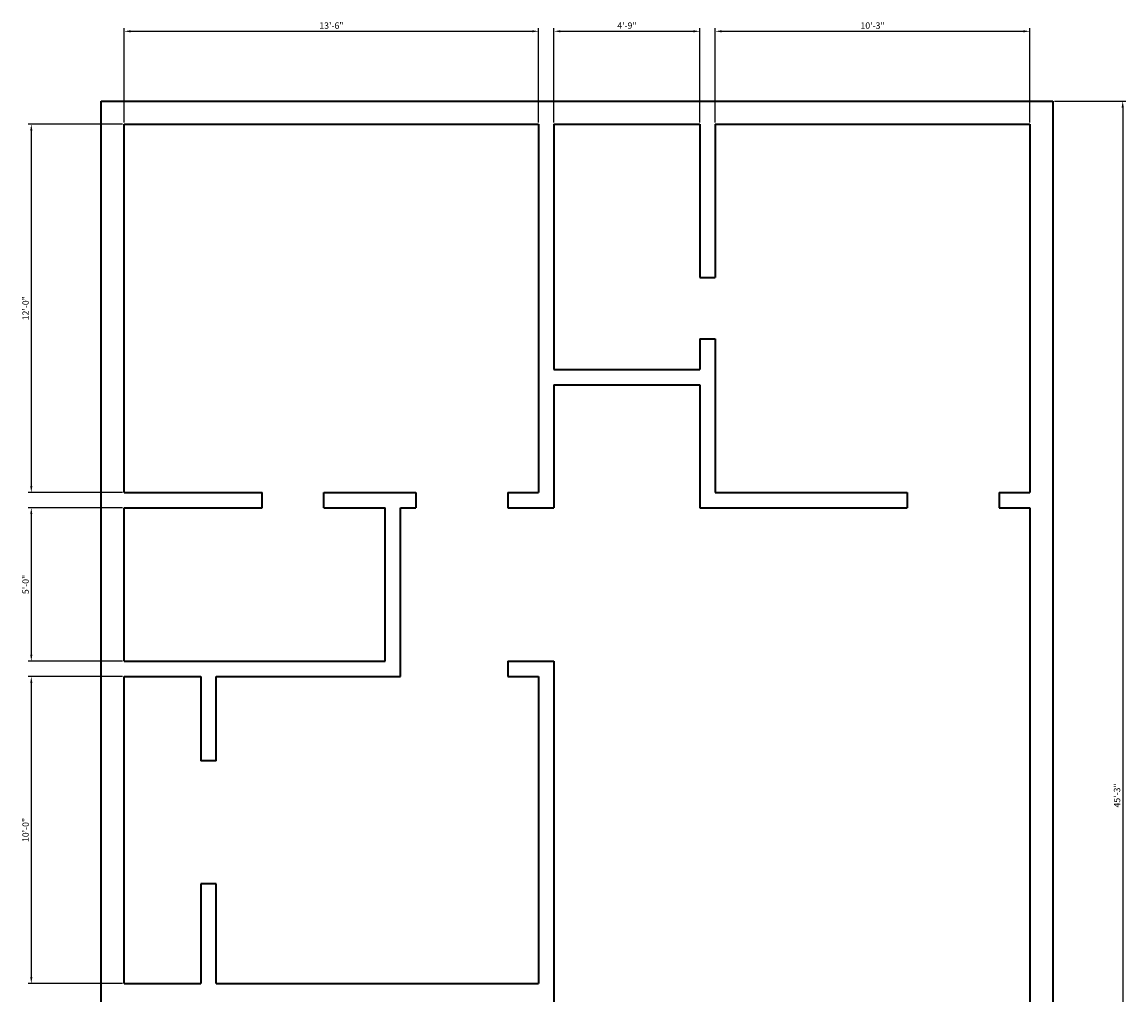
# Model space of a CAD drawing. Units: inches. Extents: x 2163 to 7246, y 928 to 2098.
# Tile 15 of 15: x 6815 to 7246, y 1625 to 2005. Entities that reach past the tile are written whole.
import ezdxf

# ---------------------------------------------------------------- set-up
doc = ezdxf.new("R2010")
doc.units = ezdxf.units.IN
doc.layers.add('A-ANNO-DIMS', color=4, linetype='Continuous', lineweight=18)
doc.layers.add('A-WALL', color=7, linetype='Continuous', lineweight=35)
doc.styles.get("Standard").update_dxf_attribs({"font": 'arial.ttf'})
doc.dimstyles.new('ISO-25', dxfattribs={"dimtxt": 2.5, "dimasz": 2.5, "dimexe": 1.25, "dimexo": 0.625, "dimtad": 1, "dimdec": 0, "dimlunit": 3, "dimtxsty": 'Standard', "dimcen": 2.5, "dimadec": 0, "dimazin": 0, "dimtfac": 1, "dimtdec": 0, "dimtmove": 0, "dimatfit": 3, "dimfxl": 1, "dimarcsym": 0})

# ---------------------------------------------------------------- blocks, each defined once
blk = doc.blocks.new('*D113')
at = {"layer": 'A-ANNO-DIMS', "color": 0, "lineweight": -2, "transparency": 16777216}
for p, q in [((7218.09, 1974.46), (7246.01, 1974.46)), ((7244.76, 1971.96), (7244.76, 1433.96)), ((7218.09, 1431.46), (7246.01, 1431.46))]:
    blk.add_line(p, q, dxfattribs=at)
at = {"layer": 'A-ANNO-DIMS', "color": 0, "transparency": 16777216}
for points in [[(7244.34, 1971.96), (7245.18, 1971.96), (7244.76, 1974.46)], [(7244.34, 1433.96), (7245.18, 1433.96), (7244.76, 1431.46)]]:
    blk.add_solid(points, dxfattribs=at)
at = {"layer": 'Defpoints', "color": 0, "transparency": 16777216}
for p in [(7217.46, 1974.46), (7217.46, 1431.46), (7244.76, 1431.46)]:
    blk.add_point(p, dxfattribs=at)
at = {"layer": 'A-ANNO-DIMS', "color": 0, "transparency": 16777216, "insert": (7242.86, 1702.96), "char_height": 2.5, "attachment_point": 5, "rotation": 90}
blk.add_mtext('45\'-3"', dxfattribs=at)
blk = doc.blocks.new('*D115')
at = {"layer": 'A-ANNO-DIMS', "color": 0, "lineweight": -2, "transparency": 16777216}
for p, q in [((6854.46, 1966.08), (6854.46, 2003.01)), ((7016.46, 1966.08), (7016.46, 2003.01)), ((6856.96, 2001.76), (7013.96, 2001.76))]:
    blk.add_line(p, q, dxfattribs=at)
at = {"layer": 'A-ANNO-DIMS', "color": 0, "transparency": 16777216}
for points in [[(6856.96, 2002.18), (6856.96, 2001.34), (6854.46, 2001.76)], [(7013.96, 2002.18), (7013.96, 2001.34), (7016.46, 2001.76)]]:
    blk.add_solid(points, dxfattribs=at)
at = {"layer": 'Defpoints', "color": 0, "transparency": 16777216}
for p in [(7016.46, 2001.76), (6854.46, 1965.46), (7016.46, 1965.46)]:
    blk.add_point(p, dxfattribs=at)
at = {"layer": 'A-ANNO-DIMS', "color": 0, "transparency": 16777216, "insert": (6935.46, 2003.66), "char_height": 2.5, "attachment_point": 5}
blk.add_mtext('13\'-6"', dxfattribs=at)
blk = doc.blocks.new('*D116')
at = {"layer": 'A-ANNO-DIMS', "color": 0, "lineweight": -2, "transparency": 16777216}
for p, q in [((7022.46, 1966.08), (7022.46, 2003.01)), ((7079.46, 1966.08), (7079.46, 2003.01)), ((7024.96, 2001.76), (7076.96, 2001.76))]:
    blk.add_line(p, q, dxfattribs=at)
at = {"layer": 'A-ANNO-DIMS', "color": 0, "transparency": 16777216}
for points in [[(7024.96, 2002.18), (7024.96, 2001.34), (7022.46, 2001.76)], [(7076.96, 2002.18), (7076.96, 2001.34), (7079.46, 2001.76)]]:
    blk.add_solid(points, dxfattribs=at)
at = {"layer": 'Defpoints', "color": 0, "transparency": 16777216}
for p in [(7079.46, 2001.76), (7022.46, 1965.46), (7079.46, 1965.46)]:
    blk.add_point(p, dxfattribs=at)
at = {"layer": 'A-ANNO-DIMS', "color": 0, "transparency": 16777216, "insert": (7050.96, 2003.66), "char_height": 2.5, "attachment_point": 5}
blk.add_mtext('4\'-9"', dxfattribs=at)
blk = doc.blocks.new('*D117')
at = {"layer": 'A-ANNO-DIMS', "color": 0, "lineweight": -2, "transparency": 16777216}
for p, q in [((7085.46, 1966.08), (7085.46, 2003.01)), ((7208.46, 1966.08), (7208.46, 2003.01)), ((7087.96, 2001.76), (7205.96, 2001.76))]:
    blk.add_line(p, q, dxfattribs=at)
at = {"layer": 'A-ANNO-DIMS', "color": 0, "transparency": 16777216}
for points in [[(7087.96, 2002.18), (7087.96, 2001.34), (7085.46, 2001.76)], [(7205.96, 2002.18), (7205.96, 2001.34), (7208.46, 2001.76)]]:
    blk.add_solid(points, dxfattribs=at)
at = {"layer": 'Defpoints', "color": 0, "transparency": 16777216}
for p in [(7208.46, 2001.76), (7085.46, 1965.46), (7208.46, 1965.46)]:
    blk.add_point(p, dxfattribs=at)
at = {"layer": 'A-ANNO-DIMS', "color": 0, "transparency": 16777216, "insert": (7146.96, 2003.66), "char_height": 2.5, "attachment_point": 5}
blk.add_mtext('10\'-3"', dxfattribs=at)
blk = doc.blocks.new('*D118')
at = {"layer": 'A-ANNO-DIMS', "color": 0, "lineweight": -2, "transparency": 16777216}
for p, q in [((6853.84, 1965.46), (6816.91, 1965.46)), ((6818.16, 1962.96), (6818.16, 1823.96)), ((6853.84, 1821.46), (6816.91, 1821.46))]:
    blk.add_line(p, q, dxfattribs=at)
at = {"layer": 'A-ANNO-DIMS', "color": 0, "transparency": 16777216}
for points in [[(6817.74, 1962.96), (6818.58, 1962.96), (6818.16, 1965.46)], [(6817.74, 1823.96), (6818.58, 1823.96), (6818.16, 1821.46)]]:
    blk.add_solid(points, dxfattribs=at)
at = {"layer": 'Defpoints', "color": 0, "transparency": 16777216}
for p in [(6854.46, 1965.46), (6818.16, 1821.46), (6854.46, 1821.46)]:
    blk.add_point(p, dxfattribs=at)
at = {"layer": 'A-ANNO-DIMS', "color": 0, "transparency": 16777216, "insert": (6816.26, 1893.46), "char_height": 2.5, "attachment_point": 5, "rotation": 90}
blk.add_mtext('12\'-0"', dxfattribs=at)
blk = doc.blocks.new('*D119')
at = {"layer": 'A-ANNO-DIMS', "color": 0, "lineweight": -2, "transparency": 16777216}
for p, q in [((6853.84, 1815.46), (6816.91, 1815.46)), ((6818.16, 1812.96), (6818.16, 1757.96)), ((6853.84, 1755.46), (6816.91, 1755.46))]:
    blk.add_line(p, q, dxfattribs=at)
at = {"layer": 'A-ANNO-DIMS', "color": 0, "transparency": 16777216}
for points in [[(6817.74, 1812.96), (6818.58, 1812.96), (6818.16, 1815.46)], [(6817.74, 1757.96), (6818.58, 1757.96), (6818.16, 1755.46)]]:
    blk.add_solid(points, dxfattribs=at)
at = {"layer": 'Defpoints', "color": 0, "transparency": 16777216}
for p in [(6854.46, 1815.46), (6818.16, 1755.46), (6854.46, 1755.46)]:
    blk.add_point(p, dxfattribs=at)
at = {"layer": 'A-ANNO-DIMS', "color": 0, "transparency": 16777216, "insert": (6816.26, 1785.46), "char_height": 2.5, "attachment_point": 5, "rotation": 90}
blk.add_mtext('5\'-0"', dxfattribs=at)
blk = doc.blocks.new('*D120')
at = {"layer": 'A-ANNO-DIMS', "color": 0, "lineweight": -2, "transparency": 16777216}
for p, q in [((6853.84, 1749.46), (6816.91, 1749.46)), ((6818.16, 1746.96), (6818.16, 1631.96)), ((6853.84, 1629.46), (6816.91, 1629.46))]:
    blk.add_line(p, q, dxfattribs=at)
at = {"layer": 'A-ANNO-DIMS', "color": 0, "transparency": 16777216}
for points in [[(6817.74, 1746.96), (6818.58, 1746.96), (6818.16, 1749.46)], [(6817.74, 1631.96), (6818.58, 1631.96), (6818.16, 1629.46)]]:
    blk.add_solid(points, dxfattribs=at)
at = {"layer": 'Defpoints', "color": 0, "transparency": 16777216}
for p in [(6854.46, 1749.46), (6818.16, 1629.46), (6854.46, 1629.46)]:
    blk.add_point(p, dxfattribs=at)
at = {"layer": 'A-ANNO-DIMS', "color": 0, "transparency": 16777216, "insert": (6816.26, 1689.46), "char_height": 2.5, "attachment_point": 5, "rotation": 90}
blk.add_mtext('10\'-0"', dxfattribs=at)

msp = doc.modelspace()

# ---------------------------------------------------------------- linework, layer by layer
at = {"layer": 'A-WALL'}
for p, q in [((6845.46, 1974.46), (7217.46, 1974.46)), ((6845.46, 1533.46), (6845.46, 1974.46)), ((7217.46, 1974.46), (7217.46, 1431.46)), ((6854.46, 1965.46), (7016.46, 1965.46)), ((6854.46, 1821.46), (6854.46, 1965.46)), ((7016.46, 1965.46), (7016.46, 1821.46)), ((7022.46, 1965.46), (7079.46, 1965.46)), ((7022.46, 1965.46), (7022.46, 1869.46)), ((7079.46, 1965.46), (7079.46, 1905.46)), ((7085.46, 1965.46), (7208.46, 1965.46)), ((7085.46, 1965.46), (7085.46, 1905.46)), ((7208.46, 1965.46), (7208.46, 1821.46)), ((7079.46, 1905.46), (7085.46, 1905.46)), ((7079.46, 1881.46), (7085.46, 1881.46)), ((7079.46, 1881.46), (7079.46, 1869.46)), ((7085.46, 1881.46), (7085.46, 1821.46)), ((7022.46, 1869.46), (7079.46, 1869.46)), ((7022.46, 1863.46), (7079.46, 1863.46)), ((7022.46, 1863.46), (7022.46, 1815.46)), ((7079.46, 1863.46), (7079.46, 1815.46)), ((6854.46, 1821.46), (6908.46, 1821.46)), ((6908.46, 1815.46), (6908.46, 1821.46)), ((6932.46, 1821.46), (6968.46, 1821.46)), ((6932.46, 1815.46), (6932.46, 1821.46)), ((6968.46, 1821.46), (6968.46, 1815.46)), ((7004.46, 1821.46), (7016.46, 1821.46)), ((7004.46, 1821.46), (7004.46, 1815.46)), ((7085.46, 1821.46), (7160.46, 1821.46)), ((7160.46, 1821.46), (7160.46, 1815.46)), ((7196.46, 1821.46), (7208.46, 1821.46)), ((7196.46, 1821.46), (7196.46, 1815.46)), ((6854.46, 1815.46), (6908.46, 1815.46)), ((6854.46, 1755.46), (6854.46, 1815.46)), ((6932.46, 1815.46), (6956.46, 1815.46)), ((6956.46, 1755.46), (6956.46, 1815.46)), ((6962.46, 1815.46), (6968.46, 1815.46)), ((6962.46, 1749.46), (6962.46, 1815.46)), ((7004.46, 1815.46), (7022.46, 1815.46)), ((7079.46, 1815.46), (7160.46, 1815.46)), ((7196.46, 1815.46), (7208.46, 1815.46)), ((7208.46, 1815.46), (7208.46, 1539.46)), ((6854.46, 1755.46), (6956.46, 1755.46)), ((7004.46, 1755.46), (7022.46, 1755.46)), ((7004.46, 1755.46), (7004.46, 1749.46)), ((7022.46, 1755.46), (7022.46, 1539.46)), ((6854.46, 1749.46), (6884.46, 1749.46)), ((6854.46, 1629.46), (6854.46, 1749.46)), ((6884.46, 1749.46), (6884.46, 1716.46)), ((6890.46, 1749.46), (6962.46, 1749.46)), ((6890.46, 1716.46), (6890.46, 1749.46)), ((7004.46, 1749.46), (7016.46, 1749.46)), ((7016.46, 1749.46), (7016.46, 1629.46)), ((6890.46, 1716.46), (6884.46, 1716.46)), ((6884.46, 1668.46), (6884.46, 1629.46)), ((6890.46, 1668.46), (6884.46, 1668.46)), ((6890.46, 1668.46), (6884.46, 1668.46)), ((6890.46, 1629.46), (6890.46, 1668.46)), ((6854.46, 1629.46), (6884.46, 1629.46)), ((6890.46, 1629.46), (7016.46, 1629.46))]:
    msp.add_line(p, q, dxfattribs=at)

# ---------------------------------------------------------------- dimensions: what is measured, and where the dimension line sits
at = {"layer": 'A-ANNO-DIMS'}
for base, p1, p2, picture, middle in [((7016.46, 2001.76), (6854.46, 1965.46), (7016.46, 1965.46), '*D115', (6935.46, 2003.66)), ((7079.46, 2001.76), (7022.46, 1965.46), (7079.46, 1965.46), '*D116', (7050.96, 2003.66)), ((7208.46, 2001.76), (7085.46, 1965.46), (7208.46, 1965.46), '*D117', (7146.96, 2003.66))]:
    dim = msp.add_linear_dim(base=base, p1=p1, p2=p2, dimstyle='ISO-25', override={"dimdec": 1, "dimlfac": 1, "dimrnd": 0, "dimzin": 1, "dimdsep": 46, "dimlunit": 4, "dimfrac": 2}, dxfattribs=at)
    dim.commit()
    dim.dimension.update_dxf_attribs({"geometry": picture, "text_midpoint": middle})
for base, p1, p2, picture, middle in [((7244.76, 1431.46), (7217.46, 1974.46), (7217.46, 1431.46), '*D113', (7242.86, 1702.96)), ((6818.16, 1821.46), (6854.46, 1965.46), (6854.46, 1821.46), '*D118', (6816.26, 1893.46)), ((6818.16, 1755.46), (6854.46, 1815.46), (6854.46, 1755.46), '*D119', (6816.26, 1785.46)), ((6818.16, 1629.46), (6854.46, 1749.46), (6854.46, 1629.46), '*D120', (6816.26, 1689.46))]:
    dim = msp.add_linear_dim(base=base, p1=p1, p2=p2, angle=90, dimstyle='ISO-25', override={"dimdec": 1, "dimlfac": 1, "dimrnd": 0, "dimzin": 1, "dimdsep": 46, "dimlunit": 4, "dimfrac": 2}, dxfattribs=at)
    dim.commit()
    dim.dimension.update_dxf_attribs({"geometry": picture, "text_midpoint": middle})

doc.saveas('drawing.dxf')
